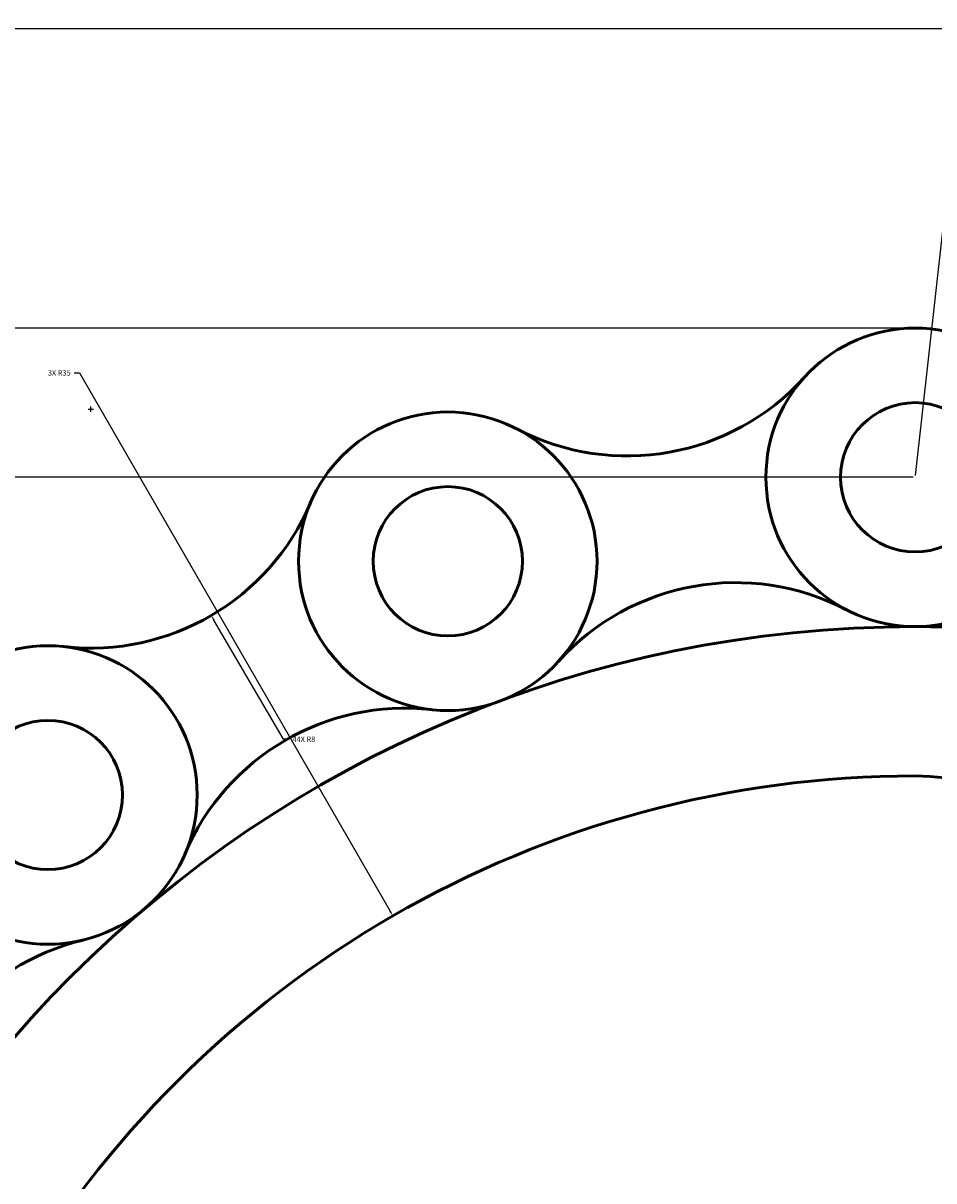
# Model space of a CAD drawing. Units: inches. Extents: x 413 to 622, y 326 to 447.
# Tile 6 of 15: x 443 to 473, y 408 to 447. Entities that reach past the tile are written whole.
import ezdxf

# ---------------------------------------------------------------- set-up
doc = ezdxf.new("R2010")
doc.units = ezdxf.units.IN
doc.header["$MEASUREMENT"] = 0
doc.layers.add('M-DIMS', color=2, linetype='Continuous', lineweight=18)
doc.layers.add('M-OUTL', color=7, linetype='Continuous', lineweight=50)
doc.styles.get("Standard").update_dxf_attribs({"font": 'arial.ttf'})
doc.dimstyles.get("Standard").update_dxf_attribs({"dimtxt": 0.18, "dimasz": 0.18, "dimexe": 0.18, "dimexo": 0.0625, "dimgap": 0.09, "dimtad": 0, "dimtih": 1, "dimtoh": 1, "dimdec": 4, "dimzin": 0, "dimdsep": 46, "dimtxsty": 'Standard', "dimcen": 0.09, "dimadec": 0, "dimazin": 0, "dimtfac": 1, "dimtdec": 4, "dimtofl": 0, "dimtmove": 0, "dimatfit": 3, "dimfxl": 1, "dimtolj": 1, "dimtzin": 0, "dimarcsym": 0})

# ---------------------------------------------------------------- blocks, each defined once
blk = doc.blocks.new('CHAIN-ROLLER-PIN')
for radius in [5, 2.5]:
    blk.add_circle((5, 5), radius)
blk = doc.blocks.new('SPROCKET-WEB-SLOT')
for centre, radius, start, end in [((7.501, 21.25), 7.5, 30, 210), ((31.317, 35), 35, 210, 270)]:
    blk.add_arc(centre, radius, start, end)
blk = doc.blocks.new('*D10')
at = {"layer": 'Defpoints', "color": 0, "transparency": 16777216}
for p in [(413.283, 436.392), (472.684, 436.392), (472.684, 336.392)]:
    blk.add_point(p, dxfattribs=at)
at = {"layer": 'M-DIMS', "color": 0, "lineweight": -2, "transparency": 16777216}
for p, q in [((472.621, 436.392), (413.103, 436.392)), ((413.283, 436.212), (413.283, 386.573)), ((413.283, 336.572), (413.283, 386.21)), ((472.621, 336.392), (413.103, 336.392))]:
    blk.add_line(p, q, dxfattribs=at)
at = {"layer": 'M-DIMS', "color": 0, "transparency": 16777216}
for points in [[(413.253, 436.212), (413.313, 436.212), (413.283, 436.392)], [(413.253, 336.572), (413.313, 336.572), (413.283, 336.392)]]:
    blk.add_solid(points, dxfattribs=at)
at = {"layer": 'M-DIMS', "color": 0, "transparency": 16777216, "insert": (413.283, 386.392), "char_height": 0.18, "attachment_point": 5}
blk.add_mtext('\\A1;100', dxfattribs=at)
blk = doc.blocks.new('*D11')
at = {"layer": 'Defpoints', "color": 0, "transparency": 16777216}
for p in [(621.66, 446.422), (621.66, 388.074), (423.314, 378.888)]:
    blk.add_point(p, dxfattribs=at)
at = {"layer": 'M-DIMS', "color": 0, "lineweight": -2, "transparency": 16777216}
for p, q in [((423.314, 378.95), (423.314, 446.602)), ((423.494, 446.422), (522.031, 446.422)), ((621.48, 446.422), (522.943, 446.422)), ((621.66, 388.137), (621.66, 446.602))]:
    blk.add_line(p, q, dxfattribs=at)
at = {"layer": 'M-DIMS', "color": 0, "transparency": 16777216}
for points in [[(423.494, 446.452), (423.494, 446.392), (423.314, 446.422)], [(621.48, 446.452), (621.48, 446.392), (621.66, 446.422)]]:
    blk.add_solid(points, dxfattribs=at)
at = {"layer": 'M-DIMS', "color": 0, "transparency": 16777216, "insert": (522.487, 446.422), "char_height": 0.18, "attachment_point": 5}
blk.add_mtext('\\A1;198.35', dxfattribs=at)
blk = doc.blocks.new('*D13')
at = {"layer": 'Defpoints', "color": 0, "transparency": 16777216}
for p in [(413.283, 431.392), (472.684, 431.392), (472.684, 386.392)]:
    blk.add_point(p, dxfattribs=at)
at = {"layer": 'M-DIMS', "color": 0, "lineweight": -2, "transparency": 16777216}
for p, q in [((472.621, 431.392), (413.103, 431.392)), ((413.283, 431.212), (413.283, 409.073)), ((413.283, 386.572), (413.283, 408.71)), ((472.621, 386.392), (413.103, 386.392))]:
    blk.add_line(p, q, dxfattribs=at)
at = {"layer": 'M-DIMS', "color": 0, "transparency": 16777216}
for points in [[(413.253, 431.212), (413.313, 431.212), (413.283, 431.392)], [(413.253, 386.572), (413.313, 386.572), (413.283, 386.392)]]:
    blk.add_solid(points, dxfattribs=at)
at = {"layer": 'M-DIMS', "color": 0, "transparency": 16777216, "insert": (413.283, 408.892), "char_height": 0.18, "attachment_point": 5}
blk.add_mtext('\\A1;45', dxfattribs=at)
blk = doc.blocks.new('*D16')
at = {"layer": 'Defpoints', "color": 0, "transparency": 16777216}
for p in [(489.47, 439.607), (472.684, 431.392), (488.355, 429.638)]:
    blk.add_point(p, dxfattribs=at)
at = {"layer": 'M-DIMS', "color": 0, "lineweight": -2, "transparency": 16777216}
for p, q in [((472.691, 431.454), (473.819, 441.539)), ((473.978, 441.34), (481.249, 440.526)), ((489.292, 439.627), (482.02, 440.44)), ((488.362, 429.7), (489.49, 439.786))]:
    blk.add_line(p, q, dxfattribs=at)
at = {"layer": 'M-DIMS', "color": 0, "transparency": 16777216}
for points in [[(473.981, 441.37), (473.974, 441.31), (473.799, 441.36)], [(489.295, 439.656), (489.288, 439.597), (489.47, 439.607)]]:
    blk.add_solid(points, dxfattribs=at)
at = {"layer": 'M-DIMS', "color": 0, "transparency": 16777216, "insert": (481.635, 440.483), "char_height": 0.18, "attachment_point": 5}
blk.add_mtext('\\A1;15.77', dxfattribs=at)
blk = doc.blocks.new('*D28')
at = {"layer": 'Defpoints', "color": 0, "transparency": 16777216}
for p in [(455.184, 416.702), (472.684, 386.392)]:
    blk.add_point(p, dxfattribs=at)
at = {"layer": 'M-DIMS', "color": 0, "lineweight": -2, "transparency": 16777216}
for p, q in [((444.504, 434.889), (444.684, 434.889)), ((444.684, 434.889), (455.094, 416.858)), ((472.594, 386.392), (472.774, 386.392)), ((472.684, 386.302), (472.684, 386.482))]:
    blk.add_line(p, q, dxfattribs=at)
at = {"layer": 'M-DIMS', "color": 0, "transparency": 16777216}
blk.add_solid([(455.12, 416.873), (455.068, 416.843), (455.184, 416.702)], dxfattribs=at)
at = {"layer": 'M-DIMS', "color": 0, "transparency": 16777216, "insert": (444.005, 434.889), "char_height": 0.18, "attachment_point": 5}
blk.add_mtext('\\A1;3X R35', dxfattribs=at)
blk = doc.blocks.new('*D33')
at = {"layer": 'Defpoints', "color": 0, "transparency": 16777216}
for p in [(445.064, 433.672), (449.1, 426.764)]:
    blk.add_point(p, dxfattribs=at)
at = {"layer": 'M-DIMS', "color": 0, "lineweight": -2, "transparency": 16777216}
for p, q in [((444.974, 433.672), (445.154, 433.672)), ((445.064, 433.582), (445.064, 433.762)), ((451.521, 422.62), (449.191, 426.609)), ((451.701, 422.62), (451.521, 422.62))]:
    blk.add_line(p, q, dxfattribs=at)
at = {"layer": 'M-DIMS', "color": 0, "transparency": 16777216}
blk.add_solid([(449.216, 426.624), (449.165, 426.594), (449.1, 426.764)], dxfattribs=at)
at = {"layer": 'M-DIMS', "color": 0, "transparency": 16777216, "insert": (452.203, 422.62), "char_height": 0.18, "attachment_point": 5}
blk.add_mtext('\\A1;44X R8', dxfattribs=at)

msp = doc.modelspace()

# ---------------------------------------------------------------- linework, layer by layer
at = {"layer": 'M-OUTL'}
msp.add_circle((472.6836, 386.3915), 40, dxfattribs=at)
for centre, start, end in [((463.037, 440.106), 242.45642, 317.90605), ((445.0645, 433.6721), 263.64571, 336.93725), ((466.6721, 419.8649), 62.45642, 137.90605), ((455.5867, 415.6593), 83.64571, 156.93725), ((446.6894, 408.1181), 103.63116, 176.58933)]:
    msp.add_arc(centre, 8, start, end, dxfattribs=at)

# ---------------------------------------------------------------- block references
for p in [(467.684, 426.392), (452.0259, 423.58), (438.6261, 415.7524)]:
    msp.add_blockref('CHAIN-ROLLER-PIN', p, dxfattribs=at)
at = {"layer": 'M-OUTL', "rotation": 239.9999999999996}
msp.add_blockref('SPROCKET-WEB-SLOT', (458.0314, 431.0122), dxfattribs=at)

# ---------------------------------------------------------------- dimensions: what is measured, and where the dimension line sits
at = {"layer": 'M-DIMS'}
dim = msp.add_linear_dim(base=(621.66, 446.422), p1=(423.3136, 378.8878), p2=(621.66, 388.0741), dimstyle='Standard', override={"dimdec": 2, "dimlfac": 1, "dimrnd": 0, "dimzin": 0, "dimdsep": 46, "dimlunit": 2}, dxfattribs=at)
dim.commit()
dim.dimension.update_dxf_attribs({"geometry": '*D11', "text_midpoint": (522.4868, 446.422)})
for base, p1, p2, angle, override, picture, middle in [((489.4705, 439.6066), (472.6836, 431.3915), (488.3553, 429.6383), 353.6169, {"dimdec": 2, "dimlfac": 1, "dimrnd": 0, "dimzin": 0, "dimdsep": 46, "dimlunit": 2}, '*D16', (481.6346, 440.4832)), ((413.2831, 436.3915), (472.6836, 336.3915), (472.6836, 436.3915), 90, {"dimdec": 0, "dimlfac": 1, "dimrnd": 0, "dimzin": 0, "dimdsep": 46, "dimlunit": 2}, '*D10', (413.2831, 386.3915)), ((413.2831, 431.3915), (472.6836, 386.3915), (472.6836, 431.3915), 90, {"dimdec": 0, "dimlfac": 1, "dimrnd": 0, "dimzin": 0, "dimdsep": 46, "dimlunit": 2}, '*D13', (413.2831, 408.8915))]:
    dim = msp.add_linear_dim(base=base, p1=p1, p2=p2, angle=angle, dimstyle='Standard', override=override, dxfattribs=at)
    dim.commit()
    dim.dimension.update_dxf_attribs({"geometry": picture, "text_midpoint": middle})
for center, mpoint, text, picture, middle in [((472.6836, 386.3915), (455.1837, 416.7025), '3X <>', '*D28', (444.0048, 434.889)), ((445.0645, 433.6721), (449.0998, 426.7644), '44X <>', '*D33', (452.2032, 422.6197))]:
    dim = msp.add_radius_dim(center=center, mpoint=mpoint, text=text, dimstyle='Standard', override={"dimdec": 0, "dimlfac": 1, "dimrnd": 0, "dimzin": 0, "dimdsep": 46, "dimlunit": 2}, dxfattribs=at)
    dim.commit()
    dim.dimension.update_dxf_attribs({"geometry": picture, "text_midpoint": middle, "dimtype": 164})

doc.saveas('drawing.dxf')
